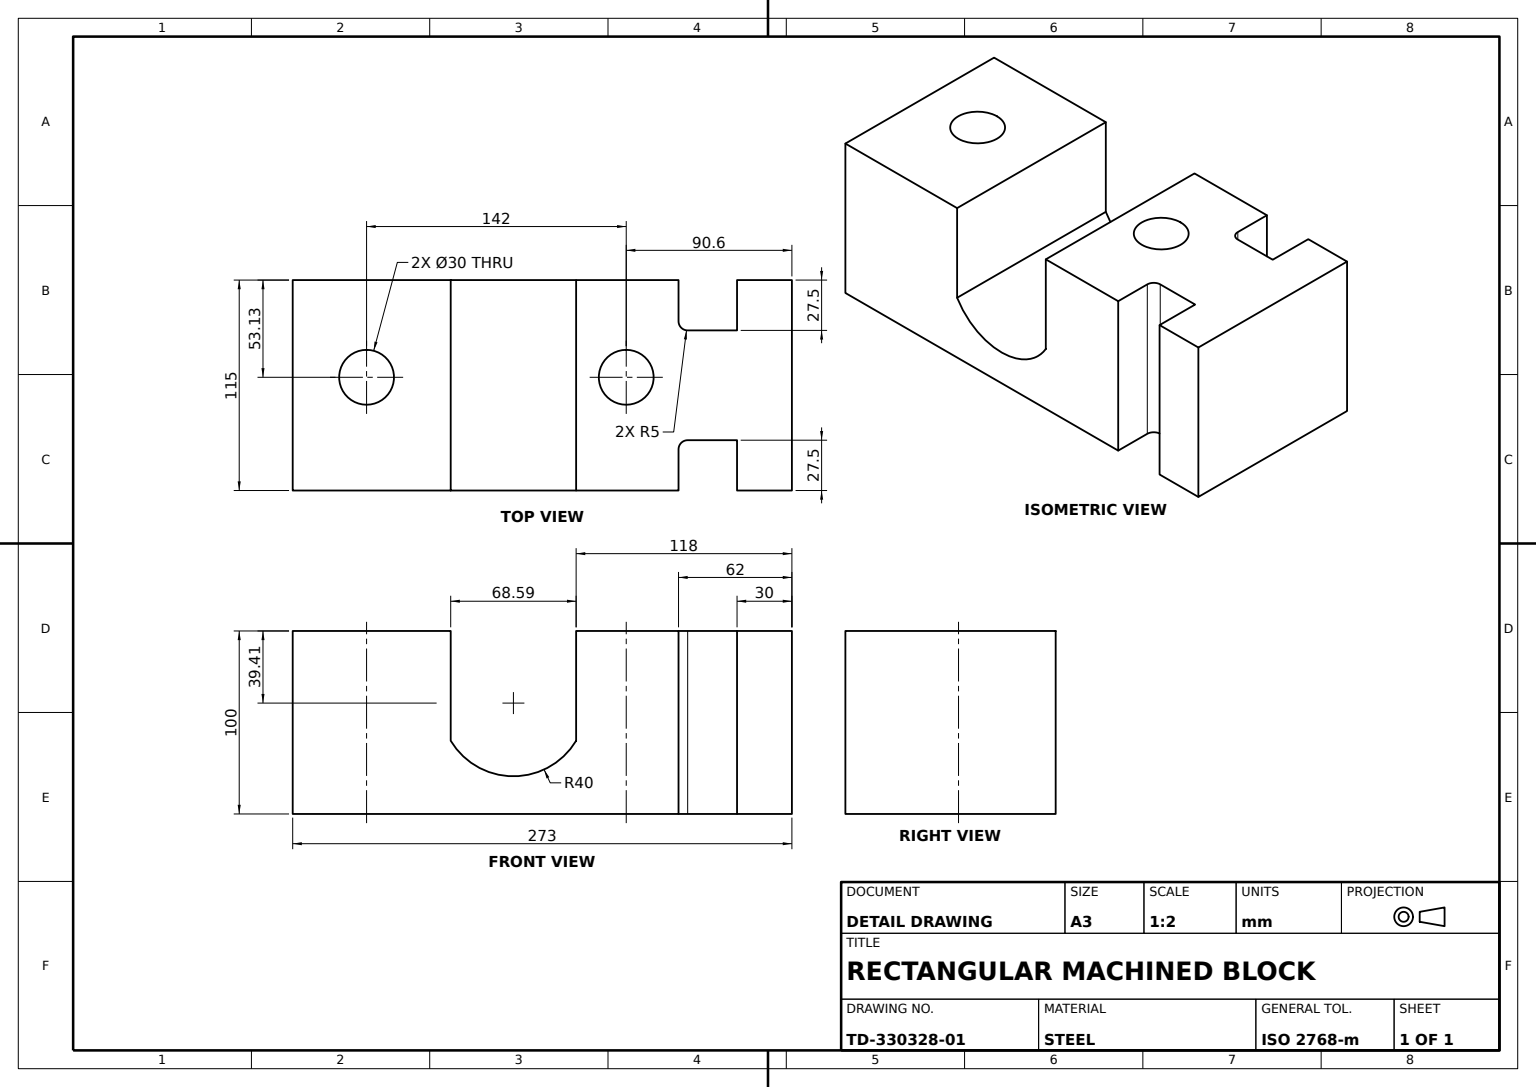
SolidWorks part; units mm, degrees
material "Plain Carbon Steel"
ref_plane "Front Plane" through (0, 0, 0) normal (0, 0, 1) x (1, 0, 0)
ref_plane "Top Plane" through (0, 0, 0) normal (0, 1, 0) x (1, 0, 0)
ref_plane "Right Plane" through (0, 0, 0) normal (1, 0, 0) x (0, 0, -1)
sketch "Support Profile Sketch" plane through (0, 0, 0) normal (0, 0, 1) x (1, 0, 0)
  line L1 (0, 0) -> (115, 0)
  line L2 (0, 0) -> (0, 30)
  line L3 (0, 30) -> (115, 30)
  line L4 (115, 0) -> (115, 30)
  line L5 (57.5, 30) -> (27.5, 30)
  line L6 (27.5, 30) -> (27.5, 57)
  line L7 (22.5, 62) -> (0, 62)
  line L8 (0, 62) -> (0, 273)
  line L9 (87.5, 30) -> (87.5, 57)
  line L10 (92.5, 62) -> (115, 62)
  line L11 (115, 62) -> (115, 273)
  arc A0 (0, 273) -> (115, 273) centre (57.5, 149.8872) cw
  arc A1 (87.5, 57) -> (92.5, 62) centre (92.5, 57) cw
  arc A2 (27.5, 57) -> (22.5, 62) centre (22.5, 57) ccw
  point P18 (87.5, 62)
  point P21 (27.5, 62)
  dimension "D1" = 5
  dimension "D2" = 135.8787
  dimension "D3" = 27.5
  dimension "D4" = 57.5
  dimension "D5" = 62
  dimension "D6" = 149.8872
extrude "Support Body" add sketch "Support Profile Sketch" along normal blind 100 contours A2 L6 L3 L9 A1 L10 L11 A0 L8 L7 | L1 L4 L3 L2
sketch "Side Mounting Holes Sketch" plane through (0, 0, 100) normal (0, 0, 1) x (1, 0, 0)
  line L0 (0, 62) -> (0, 118)
  line L1 (0, 62) -> (0, 273) construction
  line L2 (0, 118) -> (115, 118)
  line L3 (115, 62) -> (115, 273) construction
  line L4 (115, 118) -> (115, 198)
  line L5 (115, 198) -> (0, 198)
  line L6 (0, 198) -> (0, 118)
  line L7 (0, 0) -> (0, 30) construction
  line L8 (0, 0) -> (115, 0) construction
  circle A0 centre (53.1265, 232.5996) radius 15
  circle A1 centre (53.1265, 90.5996) radius 15
  dimension "D1" = 15
  dimension "D2" = 15
  dimension "D3" = 142
  dimension "D4" = 53.1265
  dimension "D5" = 90.5996
  dimension "D6" = 118
  dimension "D7" = 198
extrude "Side Mounting Holes 2x" cut sketch "Side Mounting Holes Sketch" against normal through all contours A0 | A1
sketch "Bearing Seat Sketch" plane through (0, 0, 0) normal (-1, 0, 0) x (0, 0, 1)
  line L0 (0, 273) -> (100, 273)
  line L1 (100, 273) -> (0, 273) construction
  line L2 (0, 273) -> (0, 186.5896)
  line L3 (0, 62) -> (0, 273) construction
  line L4 (0, 186.5896) -> (60, 186.5896)
  line L5 (100, 62) -> (0, 62) construction
  line L6 (60, 118) -> (0, 118)
  line L8 (100, 62) -> (100, 273) construction
  line L9 (100, 273) -> (100, 180.5)
  line L10 (100, 180.5) -> (108, 180.5)
  line L11 (100, 135.5) -> (108, 135.5)
  line L12 (108, 180.5) -> (108, 135.5)
  line L13 (100, 135.5) -> (100, 62)
  arc A0 (60, 186.5896) -> (60, 118) centre (39.412, 152.2948) cw
  dimension "D1" = 40
  dimension "D2" = 39.412
  dimension "D3" = 60
  dimension "D4" = 108
  dimension "D5" = 56
  dimension "D6" = 73.5
  dimension "D7" = 118.5
extrude "Open Bearing Seat Cut" cut sketch "Bearing Seat Sketch" against normal through all and the other way through all
